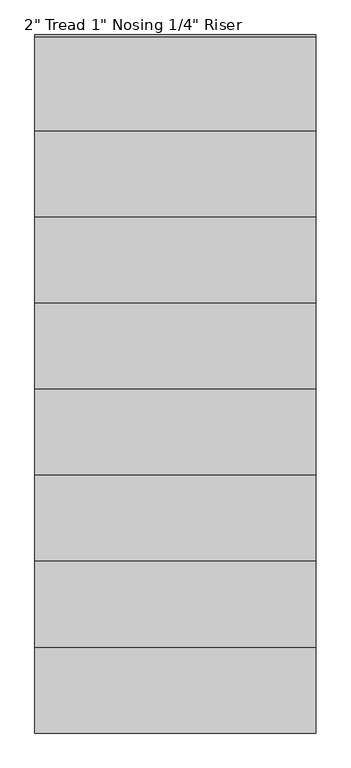
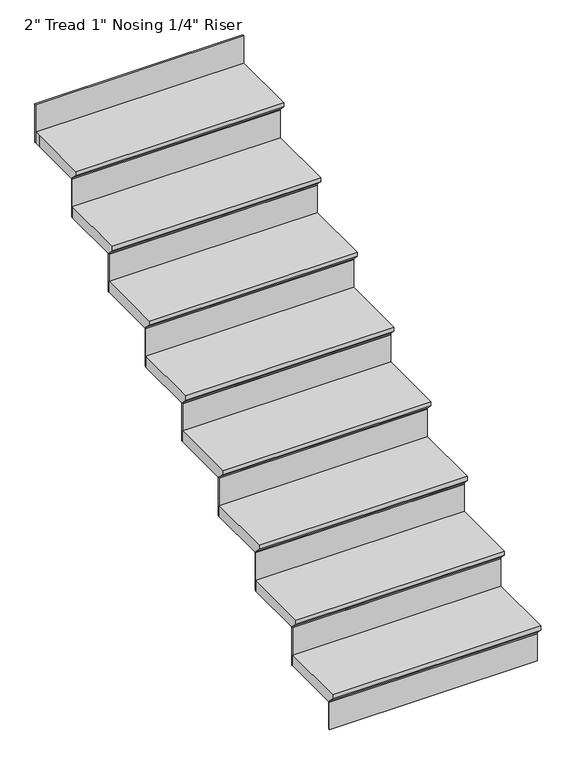
"""IFC4 building model written with IfcOpenShell, lengths in millimetres: stair flight geometry."""

from ifc_helpers import new_model, si_unit, origin, place, context, project, spatial, faceted_brep, source, transform, mapped, element, save


def stair_flight_0432408d(model_context):
    return source(origin(), model_context, "Body", "Brep", [
        faceted_brep([(-11728.968339, 6177.243496, 768.35), (-11728.968339, 6177.243496, 787.4), (-12643.368339, 6177.243496, 787.4), (-12643.368339, 6177.243496, 768.35), (-11728.968339, 6202.643496, 742.95), (-12643.368339, 6202.643496, 742.95), (-11728.968339, 6482.043496, 787.4), (-12643.368339, 6482.043496, 787.4), (-12643.368339, 6202.643496, 736.6), (-12643.368339, 6482.043496, 736.6), (-11728.968339, 6482.043496, 736.6), (-11728.968339, 6202.643496, 736.6)], [[[0, 1, 2, 3]], [[4, 0, 3, 5]], [[2, 1, 6, 7]], [[8, 9, 10, 11]], [[2, 7, 9, 8, 5, 3]], [[8, 11, 4, 5]], [[6, 1, 0, 4, 11, 10]], [[7, 6, 10, 9]]]),
        faceted_brep([(-11728.968339, 6202.643496, 736.6), (-11728.968339, 6202.643496, 609.6), (-11728.968339, 6208.993496, 609.6), (-11728.968339, 6208.993496, 736.6), (-12643.368339, 6202.643496, 736.6), (-12643.368339, 6208.993496, 736.6), (-12643.368339, 6208.993496, 609.6), (-12643.368339, 6202.643496, 609.6)], [[[0, 1, 2, 3]], [[4, 5, 6, 7]], [[1, 0, 4, 7]], [[2, 1, 7, 6]], [[3, 2, 6, 5]], [[0, 3, 5, 4]]]),
        faceted_brep([(-11728.968339, 6482.043496, 914.4), (-11728.968339, 6482.043496, 736.6), (-11728.968339, 6488.393496, 736.6), (-11728.968339, 6488.393496, 914.4), (-12643.368339, 6482.043496, 914.4), (-12643.368339, 6488.393496, 914.4), (-12643.368339, 6488.393496, 736.6), (-12643.368339, 6482.043496, 736.6)], [[[0, 1, 2, 3]], [[4, 5, 6, 7]], [[1, 0, 4, 7]], [[2, 1, 7, 6]], [[3, 2, 6, 5]], [[0, 3, 5, 4]]]),
        faceted_brep([(-12643.368339, 6456.643496, 965.2), (-11728.968339, 6456.643496, 965.2), (-11728.968339, 6761.443496, 965.2), (-12643.368339, 6761.443496, 965.2), (-12643.368339, 6482.043496, 914.4), (-12643.368339, 6761.443496, 914.4), (-11728.968339, 6761.443496, 914.4), (-11728.968339, 6482.043496, 914.4), (-12643.368339, 6482.043496, 920.75), (-12643.368339, 6456.643496, 946.15), (-11728.968339, 6482.043496, 920.75), (-11728.968339, 6456.643496, 946.15)], [[[0, 1, 2, 3]], [[4, 5, 6, 7]], [[0, 3, 5, 4, 8, 9]], [[4, 7, 10, 8]], [[2, 1, 11, 10, 7, 6]], [[3, 2, 6, 5]], [[11, 1, 0, 9]], [[10, 11, 9, 8]]]),
        faceted_brep([(-11728.968339, 6761.443496, 1092.2), (-11728.968339, 6761.443496, 914.4), (-11728.968339, 6767.793496, 914.4), (-11728.968339, 6767.793496, 1092.2), (-12643.368339, 6761.443496, 1092.2), (-12643.368339, 6767.793496, 1092.2), (-12643.368339, 6767.793496, 914.4), (-12643.368339, 6761.443496, 914.4)], [[[0, 1, 2, 3]], [[4, 5, 6, 7]], [[1, 0, 4, 7]], [[2, 1, 7, 6]], [[3, 2, 6, 5]], [[0, 3, 5, 4]]]),
        faceted_brep([(-12643.368339, 6736.043496, 1143.0), (-11728.968339, 6736.043496, 1143.0), (-11728.968339, 7040.843496, 1143.0), (-12643.368339, 7040.843496, 1143.0), (-12643.368339, 6761.443496, 1092.2), (-12643.368339, 7040.843496, 1092.2), (-11728.968339, 7040.843496, 1092.2), (-11728.968339, 6761.443496, 1092.2), (-12643.368339, 6761.443496, 1098.55), (-12643.368339, 6736.043496, 1123.95), (-11728.968339, 6761.443496, 1098.55), (-11728.968339, 6736.043496, 1123.95)], [[[0, 1, 2, 3]], [[4, 5, 6, 7]], [[0, 3, 5, 4, 8, 9]], [[4, 7, 10, 8]], [[2, 1, 11, 10, 7, 6]], [[3, 2, 6, 5]], [[11, 1, 0, 9]], [[10, 11, 9, 8]]]),
        faceted_brep([(-11728.968339, 7040.843496, 1270.0), (-11728.968339, 7040.843496, 1092.2), (-11728.968339, 7047.193496, 1092.2), (-11728.968339, 7047.193496, 1270.0), (-12643.368339, 7040.843496, 1270.0), (-12643.368339, 7047.193496, 1270.0), (-12643.368339, 7047.193496, 1092.2), (-12643.368339, 7040.843496, 1092.2)], [[[0, 1, 2, 3]], [[4, 5, 6, 7]], [[1, 0, 4, 7]], [[2, 1, 7, 6]], [[3, 2, 6, 5]], [[0, 3, 5, 4]]]),
        faceted_brep([(-12643.368339, 7015.443496, 1320.8), (-11728.968339, 7015.443496, 1320.8), (-11728.968339, 7320.243496, 1320.8), (-12643.368339, 7320.243496, 1320.8), (-12643.368339, 7040.843496, 1270.0), (-12643.368339, 7320.243496, 1270.0), (-11728.968339, 7320.243496, 1270.0), (-11728.968339, 7040.843496, 1270.0), (-12643.368339, 7040.843496, 1276.35), (-12643.368339, 7015.443496, 1301.75), (-11728.968339, 7040.843496, 1276.35), (-11728.968339, 7015.443496, 1301.75)], [[[0, 1, 2, 3]], [[4, 5, 6, 7]], [[0, 3, 5, 4, 8, 9]], [[4, 7, 10, 8]], [[2, 1, 11, 10, 7, 6]], [[3, 2, 6, 5]], [[11, 1, 0, 9]], [[10, 11, 9, 8]]]),
        faceted_brep([(-11728.968339, 7320.243496, 1447.8), (-11728.968339, 7320.243496, 1270.0), (-11728.968339, 7326.593496, 1270.0), (-11728.968339, 7326.593496, 1447.8), (-12643.368339, 7320.243496, 1447.8), (-12643.368339, 7326.593496, 1447.8), (-12643.368339, 7326.593496, 1270.0), (-12643.368339, 7320.243496, 1270.0)], [[[0, 1, 2, 3]], [[4, 5, 6, 7]], [[1, 0, 4, 7]], [[2, 1, 7, 6]], [[3, 2, 6, 5]], [[0, 3, 5, 4]]]),
        faceted_brep([(-12643.368339, 7294.843496, 1498.6), (-11728.968339, 7294.843496, 1498.6), (-11728.968339, 7599.643496, 1498.6), (-12643.368339, 7599.643496, 1498.6), (-12643.368339, 7320.243496, 1447.8), (-12643.368339, 7599.643496, 1447.8), (-11728.968339, 7599.643496, 1447.8), (-11728.968339, 7320.243496, 1447.8), (-12643.368339, 7320.243496, 1454.15), (-12643.368339, 7294.843496, 1479.55), (-11728.968339, 7320.243496, 1454.15), (-11728.968339, 7294.843496, 1479.55)], [[[0, 1, 2, 3]], [[4, 5, 6, 7]], [[0, 3, 5, 4, 8, 9]], [[4, 7, 10, 8]], [[2, 1, 11, 10, 7, 6]], [[3, 2, 6, 5]], [[11, 1, 0, 9]], [[10, 11, 9, 8]]]),
        faceted_brep([(-11728.968339, 7599.643496, 1625.6), (-11728.968339, 7599.643496, 1447.8), (-11728.968339, 7605.993496, 1447.8), (-11728.968339, 7605.993496, 1625.6), (-12643.368339, 7599.643496, 1625.6), (-12643.368339, 7605.993496, 1625.6), (-12643.368339, 7605.993496, 1447.8), (-12643.368339, 7599.643496, 1447.8)], [[[0, 1, 2, 3]], [[4, 5, 6, 7]], [[1, 0, 4, 7]], [[2, 1, 7, 6]], [[3, 2, 6, 5]], [[0, 3, 5, 4]]]),
        faceted_brep([(-12643.368339, 7574.243496, 1676.4), (-11728.968339, 7574.243496, 1676.4), (-11728.968339, 7879.043496, 1676.4), (-12643.368339, 7879.043496, 1676.4), (-12643.368339, 7599.643496, 1625.6), (-12643.368339, 7879.043496, 1625.6), (-11728.968339, 7879.043496, 1625.6), (-11728.968339, 7599.643496, 1625.6), (-12643.368339, 7599.643496, 1631.95), (-12643.368339, 7574.243496, 1657.35), (-11728.968339, 7599.643496, 1631.95), (-11728.968339, 7574.243496, 1657.35)], [[[0, 1, 2, 3]], [[4, 5, 6, 7]], [[0, 3, 5, 4, 8, 9]], [[4, 7, 10, 8]], [[2, 1, 11, 10, 7, 6]], [[3, 2, 6, 5]], [[11, 1, 0, 9]], [[10, 11, 9, 8]]]),
        faceted_brep([(-11728.968339, 7879.043496, 1803.4), (-11728.968339, 7879.043496, 1625.6), (-11728.968339, 7885.393496, 1625.6), (-11728.968339, 7885.393496, 1803.4), (-12643.368339, 7879.043496, 1803.4), (-12643.368339, 7885.393496, 1803.4), (-12643.368339, 7885.393496, 1625.6), (-12643.368339, 7879.043496, 1625.6)], [[[0, 1, 2, 3]], [[4, 5, 6, 7]], [[1, 0, 4, 7]], [[2, 1, 7, 6]], [[3, 2, 6, 5]], [[0, 3, 5, 4]]]),
        faceted_brep([(-12643.368339, 7853.643496, 1854.2), (-11728.968339, 7853.643496, 1854.2), (-11728.968339, 8158.443496, 1854.2), (-12643.368339, 8158.443496, 1854.2), (-12643.368339, 7879.043496, 1803.4), (-12643.368339, 8158.443496, 1803.4), (-11728.968339, 8158.443496, 1803.4), (-11728.968339, 7879.043496, 1803.4), (-12643.368339, 7879.043496, 1809.75), (-12643.368339, 7853.643496, 1835.15), (-11728.968339, 7879.043496, 1809.75), (-11728.968339, 7853.643496, 1835.15)], [[[0, 1, 2, 3]], [[4, 5, 6, 7]], [[0, 3, 5, 4, 8, 9]], [[4, 7, 10, 8]], [[2, 1, 11, 10, 7, 6]], [[3, 2, 6, 5]], [[11, 1, 0, 9]], [[10, 11, 9, 8]]]),
        faceted_brep([(-11728.968339, 8437.843496, 2159.0), (-11728.968339, 8437.843496, 1981.2), (-11728.968339, 8444.193496, 1981.2), (-11728.968339, 8444.193496, 2159.0), (-12643.368339, 8437.843496, 2159.0), (-12643.368339, 8444.193496, 2159.0), (-12643.368339, 8444.193496, 1981.2), (-12643.368339, 8437.843496, 1981.2)], [[[0, 1, 2, 3]], [[4, 5, 6, 7]], [[1, 0, 4, 7]], [[2, 1, 7, 6]], [[3, 2, 6, 5]], [[0, 3, 5, 4]]]),
        faceted_brep([(-11728.968339, 8158.443496, 1981.2), (-11728.968339, 8158.443496, 1803.4), (-11728.968339, 8164.793496, 1803.4), (-11728.968339, 8164.793496, 1981.2), (-12643.368339, 8158.443496, 1981.2), (-12643.368339, 8164.793496, 1981.2), (-12643.368339, 8164.793496, 1803.4), (-12643.368339, 8158.443496, 1803.4)], [[[0, 1, 2, 3]], [[4, 5, 6, 7]], [[1, 0, 4, 7]], [[2, 1, 7, 6]], [[3, 2, 6, 5]], [[0, 3, 5, 4]]]),
        faceted_brep([(-12643.368339, 8437.843496, 2032.0), (-12643.368339, 8412.443496, 2032.0), (-12643.368339, 8133.043496, 2032.0), (-11728.968339, 8133.043496, 2032.0), (-11728.968339, 8437.843496, 2032.0), (-12643.368339, 8412.443496, 1981.2), (-12643.368339, 8437.843496, 1981.2), (-11728.968339, 8437.843496, 1981.2), (-11728.968339, 8158.443496, 1981.2), (-12643.368339, 8158.443496, 1981.2), (-12643.368339, 8158.443496, 1987.55), (-12643.368339, 8133.043496, 2012.95), (-11728.968339, 8158.443496, 1987.55), (-11728.968339, 8133.043496, 2012.95)], [[[0, 1, 2, 3, 4]], [[5, 6, 7, 8, 9]], [[1, 0, 6, 5]], [[2, 1, 5, 9, 10, 11]], [[9, 8, 12, 10]], [[4, 3, 13, 12, 8, 7]], [[0, 4, 7, 6]], [[13, 3, 2, 11]], [[12, 13, 11, 10]]]),
    ])


if __name__ == "__main__":
    model = new_model("IFC4")
    model_context = context("Model", 3, world=origin())
    ifc_project = project(units=[si_unit("LENGTHUNIT", "METRE", prefix="MILLI")], contexts=[model_context])
    site = spatial("IfcSite", under=ifc_project)
    building = spatial("IfcBuilding", under=site)
    placement = place(None, origin())
    stair_flight_shape = stair_flight_0432408d(model_context)
    element("IfcStairFlight", 1, ObjectType="2\" Tread 1\" Nosing 1/4\" Riser", at=placement, inside=building, context=model_context, shape_type="MappedRepresentation", body=[
        mapped(stair_flight_shape, transform((0.0, 0.0, 0.0), x_axis=(1.0, 0.0, 0.0), y_axis=(0.0, 1.0, 0.0), z_axis=(0.0, 0.0, 1.0))),
    ])
    save(model, "model.ifc")
